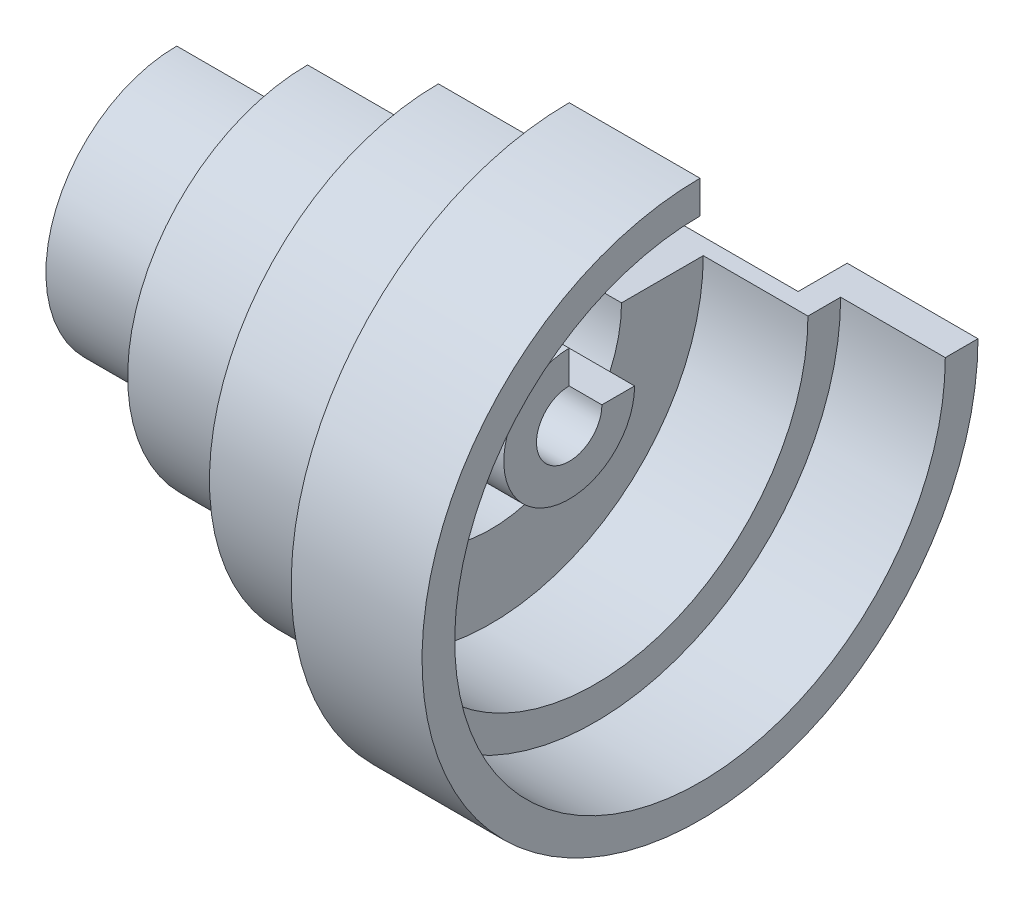
ISO-10303-21;
HEADER;
FILE_DESCRIPTION(('STEP AP214'),'2;1');
FILE_NAME('part.step','',(''),(''),'','','');
FILE_SCHEMA(('AUTOMOTIVE_DESIGN { 1 0 10303 214 1 1 1 1 }'));
ENDSEC;
DATA;
#1=APPLICATION_CONTEXT('core data for automotive mechanical design processes');
#2=APPLICATION_PROTOCOL_DEFINITION('international standard','automotive_design',2000,#1);
#3=PRODUCT_CONTEXT('',#1,'mechanical');
#4=PRODUCT('Part','Part','',(#3));
#5=PRODUCT_RELATED_PRODUCT_CATEGORY('part','',(#4));
#6=PRODUCT_DEFINITION_FORMATION('','',#4);
#7=PRODUCT_DEFINITION_CONTEXT('part definition',#1,'design');
#8=PRODUCT_DEFINITION('design','',#6,#7);
#9=PRODUCT_DEFINITION_SHAPE('','',#8);
#10=(LENGTH_UNIT() NAMED_UNIT(*) SI_UNIT(.MILLI.,.METRE.));
#11=(NAMED_UNIT(*) PLANE_ANGLE_UNIT() SI_UNIT($,.RADIAN.));
#12=(NAMED_UNIT(*) SI_UNIT($,.STERADIAN.) SOLID_ANGLE_UNIT());
#13=UNCERTAINTY_MEASURE_WITH_UNIT(LENGTH_MEASURE(1.E-05),#10,'distance_accuracy_value','');
#14=(GEOMETRIC_REPRESENTATION_CONTEXT(3) GLOBAL_UNCERTAINTY_ASSIGNED_CONTEXT((#13)) GLOBAL_UNIT_ASSIGNED_CONTEXT((#10,
#11,#12)) REPRESENTATION_CONTEXT('',''));
#15=CARTESIAN_POINT('',(0.,0.,0.));
#16=DIRECTION('',(0.,0.,1.));
#17=DIRECTION('',(1.,0.,0.));
#18=AXIS2_PLACEMENT_3D('',#15,#16,#17);
#19=CARTESIAN_POINT('',(0.,0.,0.));
#20=DIRECTION('',(-1.,0.,0.));
#21=DIRECTION('',(0.,0.,1.));
#22=AXIS2_PLACEMENT_3D('',#19,#20,#21);
#23=CYLINDRICAL_SURFACE('',#22,10.);
#24=CARTESIAN_POINT('',(120.,0.,0.));
#25=DIRECTION('',(-1.,0.,0.));
#26=DIRECTION('',(0.,0.,1.));
#27=AXIS2_PLACEMENT_3D('',#24,#25,#26);
#28=CIRCLE('',#27,10.);
#29=CARTESIAN_POINT('',(120.,1.04744440165294E-13,-10.));
#30=VERTEX_POINT('',#29);
#31=CARTESIAN_POINT('',(120.,10.,0.));
#32=VERTEX_POINT('',#31);
#33=EDGE_CURVE('E11',#30,#32,#28,.T.);
#34=ORIENTED_EDGE('',*,*,#33,.F.);
#35=DIRECTION('',(-1.,0.,0.));
#36=VECTOR('',#35,1.);
#37=CARTESIAN_POINT('',(0.,1.04744440165294E-13,-10.));
#38=LINE('',#37,#36);
#39=CARTESIAN_POINT('',(0.,1.04744440165294E-13,-10.));
#40=VERTEX_POINT('',#39);
#41=EDGE_CURVE('E228',#30,#40,#38,.T.);
#42=ORIENTED_EDGE('',*,*,#41,.T.);
#43=CARTESIAN_POINT('',(0.,0.,0.));
#44=DIRECTION('',(-1.,0.,0.));
#45=DIRECTION('',(0.,0.,1.));
#46=AXIS2_PLACEMENT_3D('',#43,#44,#45);
#47=CIRCLE('',#46,10.);
#48=CARTESIAN_POINT('',(0.,10.,0.));
#49=VERTEX_POINT('',#48);
#50=EDGE_CURVE('E57',#40,#49,#47,.T.);
#51=ORIENTED_EDGE('',*,*,#50,.T.);
#52=DIRECTION('',(-1.,0.,0.));
#53=VECTOR('',#52,1.);
#54=CARTESIAN_POINT('',(0.,10.,0.));
#55=LINE('',#54,#53);
#56=EDGE_CURVE('E178',#32,#49,#55,.T.);
#57=ORIENTED_EDGE('',*,*,#56,.F.);
#58=EDGE_LOOP('',(#34,#42,#51,#57));
#59=FACE_BOUND('',#58,.T.);
#60=ADVANCED_FACE('F41',(#59),#23,.F.);
#61=CARTESIAN_POINT('',(120.,0.,0.));
#62=DIRECTION('',(1.,0.,0.));
#63=DIRECTION('',(0.,0.,-1.));
#64=AXIS2_PLACEMENT_3D('',#61,#62,#63);
#65=PLANE('',#64);
#66=CARTESIAN_POINT('',(120.,0.,0.));
#67=DIRECTION('',(-1.,0.,0.));
#68=DIRECTION('',(0.,0.,1.));
#69=AXIS2_PLACEMENT_3D('',#66,#67,#68);
#70=CIRCLE('',#69,20.);
#71=CARTESIAN_POINT('',(120.,2.09488880330588E-13,-20.));
#72=VERTEX_POINT('',#71);
#73=CARTESIAN_POINT('',(120.,20.,0.));
#74=VERTEX_POINT('',#73);
#75=EDGE_CURVE('E47',#72,#74,#70,.T.);
#76=ORIENTED_EDGE('',*,*,#75,.F.);
#77=DIRECTION('',(0.,0.,1.));
#78=VECTOR('',#77,1.);
#79=CARTESIAN_POINT('',(120.,0.,0.));
#80=LINE('',#79,#78);
#81=EDGE_CURVE('E175',#72,#30,#80,.T.);
#82=ORIENTED_EDGE('',*,*,#81,.T.);
#83=ORIENTED_EDGE('',*,*,#33,.T.);
#84=DIRECTION('',(0.,-1.,0.));
#85=VECTOR('',#84,1.);
#86=CARTESIAN_POINT('',(120.,0.,0.));
#87=LINE('',#86,#85);
#88=EDGE_CURVE('E166',#74,#32,#87,.T.);
#89=ORIENTED_EDGE('',*,*,#88,.F.);
#90=EDGE_LOOP('',(#76,#82,#83,#89));
#91=FACE_BOUND('',#90,.T.);
#92=ADVANCED_FACE('F43',(#91),#65,.T.);
#93=CARTESIAN_POINT('',(0.,0.,0.));
#94=DIRECTION('',(-1.,0.,0.));
#95=DIRECTION('',(0.,0.,1.));
#96=AXIS2_PLACEMENT_3D('',#93,#94,#95);
#97=CYLINDRICAL_SURFACE('',#96,20.);
#98=CARTESIAN_POINT('',(63.9999999999999,0.,0.));
#99=DIRECTION('',(-1.,0.,0.));
#100=DIRECTION('',(0.,0.,1.));
#101=AXIS2_PLACEMENT_3D('',#98,#99,#100);
#102=CIRCLE('',#101,20.);
#103=CARTESIAN_POINT('',(63.9999999999999,2.09488880330588E-13,-20.));
#104=VERTEX_POINT('',#103);
#105=CARTESIAN_POINT('',(63.9999999999999,20.,0.));
#106=VERTEX_POINT('',#105);
#107=EDGE_CURVE('E307',#104,#106,#102,.T.);
#108=ORIENTED_EDGE('',*,*,#107,.F.);
#109=DIRECTION('',(1.,0.,0.));
#110=VECTOR('',#109,1.);
#111=CARTESIAN_POINT('',(0.,2.09488880330588E-13,-20.));
#112=LINE('',#111,#110);
#113=EDGE_CURVE('E232',#104,#72,#112,.T.);
#114=ORIENTED_EDGE('',*,*,#113,.T.);
#115=ORIENTED_EDGE('',*,*,#75,.T.);
#116=DIRECTION('',(1.,0.,0.));
#117=VECTOR('',#116,1.);
#118=CARTESIAN_POINT('',(0.,20.,0.));
#119=LINE('',#118,#117);
#120=EDGE_CURVE('E181',#106,#74,#119,.T.);
#121=ORIENTED_EDGE('',*,*,#120,.F.);
#122=EDGE_LOOP('',(#108,#114,#115,#121));
#123=FACE_BOUND('',#122,.T.);
#124=ADVANCED_FACE('F310',(#123),#97,.T.);
#125=CARTESIAN_POINT('',(63.9999999999999,0.,0.));
#126=DIRECTION('',(1.,0.,0.));
#127=DIRECTION('',(0.,0.,-1.));
#128=AXIS2_PLACEMENT_3D('',#125,#126,#127);
#129=PLANE('',#128);
#130=CARTESIAN_POINT('',(63.9999999999999,0.,0.));
#131=DIRECTION('',(-1.,0.,0.));
#132=DIRECTION('',(0.,0.,1.));
#133=AXIS2_PLACEMENT_3D('',#130,#131,#132);
#134=CIRCLE('',#133,40.);
#135=CARTESIAN_POINT('',(63.9999999999999,4.18977760661176E-13,-40.));
#136=VERTEX_POINT('',#135);
#137=CARTESIAN_POINT('',(63.9999999999999,40.,0.));
#138=VERTEX_POINT('',#137);
#139=EDGE_CURVE('E301',#136,#138,#134,.T.);
#140=ORIENTED_EDGE('',*,*,#139,.F.);
#141=DIRECTION('',(0.,0.,1.));
#142=VECTOR('',#141,1.);
#143=CARTESIAN_POINT('',(63.9999999999999,0.,0.));
#144=LINE('',#143,#142);
#145=EDGE_CURVE('E237',#136,#104,#144,.T.);
#146=ORIENTED_EDGE('',*,*,#145,.T.);
#147=ORIENTED_EDGE('',*,*,#107,.T.);
#148=DIRECTION('',(0.,-1.,0.));
#149=VECTOR('',#148,1.);
#150=CARTESIAN_POINT('',(63.9999999999999,0.,0.));
#151=LINE('',#150,#149);
#152=EDGE_CURVE('E183',#138,#106,#151,.T.);
#153=ORIENTED_EDGE('',*,*,#152,.F.);
#154=EDGE_LOOP('',(#140,#146,#147,#153));
#155=FACE_BOUND('',#154,.T.);
#156=ADVANCED_FACE('F370',(#155),#129,.T.);
#157=CARTESIAN_POINT('',(0.,0.,0.));
#158=DIRECTION('',(-1.,0.,0.));
#159=DIRECTION('',(0.,0.,1.));
#160=AXIS2_PLACEMENT_3D('',#157,#158,#159);
#161=CYLINDRICAL_SURFACE('',#160,40.);
#162=CARTESIAN_POINT('',(95.9999999999999,0.,0.));
#163=DIRECTION('',(-1.,0.,0.));
#164=DIRECTION('',(0.,0.,1.));
#165=AXIS2_PLACEMENT_3D('',#162,#163,#164);
#166=CIRCLE('',#165,40.);
#167=CARTESIAN_POINT('',(95.9999999999999,4.18977760661176E-13,-40.));
#168=VERTEX_POINT('',#167);
#169=CARTESIAN_POINT('',(95.9999999999999,40.,0.));
#170=VERTEX_POINT('',#169);
#171=EDGE_CURVE('E302',#168,#170,#166,.T.);
#172=ORIENTED_EDGE('',*,*,#171,.F.);
#173=DIRECTION('',(-1.,0.,0.));
#174=VECTOR('',#173,1.);
#175=CARTESIAN_POINT('',(0.,4.18977760661176E-13,-40.));
#176=LINE('',#175,#174);
#177=EDGE_CURVE('E239',#168,#136,#176,.T.);
#178=ORIENTED_EDGE('',*,*,#177,.T.);
#179=ORIENTED_EDGE('',*,*,#139,.T.);
#180=DIRECTION('',(-1.,0.,0.));
#181=VECTOR('',#180,1.);
#182=CARTESIAN_POINT('',(0.,40.,0.));
#183=LINE('',#182,#181);
#184=EDGE_CURVE('E186',#170,#138,#183,.T.);
#185=ORIENTED_EDGE('',*,*,#184,.F.);
#186=EDGE_LOOP('',(#172,#178,#179,#185));
#187=FACE_BOUND('',#186,.T.);
#188=ADVANCED_FACE('F365',(#187),#161,.F.);
#189=CARTESIAN_POINT('',(95.9999999999999,0.,0.));
#190=DIRECTION('',(1.,0.,0.));
#191=DIRECTION('',(0.,0.,-1.));
#192=AXIS2_PLACEMENT_3D('',#189,#190,#191);
#193=PLANE('',#192);
#194=CARTESIAN_POINT('',(95.9999999999999,0.,0.));
#195=DIRECTION('',(-1.,0.,0.));
#196=DIRECTION('',(0.,0.,1.));
#197=AXIS2_PLACEMENT_3D('',#194,#195,#196);
#198=CIRCLE('',#197,65.);
#199=CARTESIAN_POINT('',(95.9999999999999,6.80838861074411E-13,-65.));
#200=VERTEX_POINT('',#199);
#201=CARTESIAN_POINT('',(95.9999999999999,65.,0.));
#202=VERTEX_POINT('',#201);
#203=EDGE_CURVE('E303',#200,#202,#198,.T.);
#204=ORIENTED_EDGE('',*,*,#203,.F.);
#205=DIRECTION('',(0.,0.,1.));
#206=VECTOR('',#205,1.);
#207=CARTESIAN_POINT('',(95.9999999999999,0.,0.));
#208=LINE('',#207,#206);
#209=EDGE_CURVE('E245',#200,#168,#208,.T.);
#210=ORIENTED_EDGE('',*,*,#209,.T.);
#211=ORIENTED_EDGE('',*,*,#171,.T.);
#212=DIRECTION('',(0.,-1.,0.));
#213=VECTOR('',#212,1.);
#214=CARTESIAN_POINT('',(95.9999999999999,0.,0.));
#215=LINE('',#214,#213);
#216=EDGE_CURVE('E194',#202,#170,#215,.T.);
#217=ORIENTED_EDGE('',*,*,#216,.F.);
#218=EDGE_LOOP('',(#204,#210,#211,#217));
#219=FACE_BOUND('',#218,.T.);
#220=ADVANCED_FACE('F356',(#219),#193,.T.);
#221=CARTESIAN_POINT('',(0.,0.,0.));
#222=DIRECTION('',(-1.,0.,0.));
#223=DIRECTION('',(0.,0.,1.));
#224=AXIS2_PLACEMENT_3D('',#221,#222,#223);
#225=CYLINDRICAL_SURFACE('',#224,65.);
#226=CARTESIAN_POINT('',(128.,0.,0.));
#227=DIRECTION('',(-1.,0.,0.));
#228=DIRECTION('',(0.,0.,1.));
#229=AXIS2_PLACEMENT_3D('',#226,#227,#228);
#230=CIRCLE('',#229,65.);
#231=CARTESIAN_POINT('',(128.,6.80838861074411E-13,-65.));
#232=VERTEX_POINT('',#231);
#233=CARTESIAN_POINT('',(128.,65.,0.));
#234=VERTEX_POINT('',#233);
#235=EDGE_CURVE('E296',#232,#234,#230,.T.);
#236=ORIENTED_EDGE('',*,*,#235,.F.);
#237=DIRECTION('',(-1.,0.,0.));
#238=VECTOR('',#237,1.);
#239=CARTESIAN_POINT('',(0.,6.80838861074411E-13,-65.));
#240=LINE('',#239,#238);
#241=EDGE_CURVE('E243',#232,#200,#240,.T.);
#242=ORIENTED_EDGE('',*,*,#241,.T.);
#243=ORIENTED_EDGE('',*,*,#203,.T.);
#244=DIRECTION('',(-1.,0.,0.));
#245=VECTOR('',#244,1.);
#246=CARTESIAN_POINT('',(0.,65.,0.));
#247=LINE('',#246,#245);
#248=EDGE_CURVE('E191',#234,#202,#247,.T.);
#249=ORIENTED_EDGE('',*,*,#248,.F.);
#250=EDGE_LOOP('',(#236,#242,#243,#249));
#251=FACE_BOUND('',#250,.T.);
#252=ADVANCED_FACE('F358',(#251),#225,.F.);
#253=CARTESIAN_POINT('',(128.,0.,0.));
#254=DIRECTION('',(1.,0.,0.));
#255=DIRECTION('',(0.,0.,-1.));
#256=AXIS2_PLACEMENT_3D('',#253,#254,#255);
#257=PLANE('',#256);
#258=CARTESIAN_POINT('',(128.,0.,0.));
#259=DIRECTION('',(-1.,0.,0.));
#260=DIRECTION('',(0.,0.,1.));
#261=AXIS2_PLACEMENT_3D('',#258,#259,#260);
#262=CIRCLE('',#261,75.);
#263=CARTESIAN_POINT('',(128.,7.85583301239705E-13,-75.));
#264=VERTEX_POINT('',#263);
#265=CARTESIAN_POINT('',(128.,75.,0.));
#266=VERTEX_POINT('',#265);
#267=EDGE_CURVE('E300',#264,#266,#262,.T.);
#268=ORIENTED_EDGE('',*,*,#267,.F.);
#269=DIRECTION('',(0.,0.,1.));
#270=VECTOR('',#269,1.);
#271=CARTESIAN_POINT('',(128.,0.,0.));
#272=LINE('',#271,#270);
#273=EDGE_CURVE('E247',#264,#232,#272,.T.);
#274=ORIENTED_EDGE('',*,*,#273,.T.);
#275=ORIENTED_EDGE('',*,*,#235,.T.);
#276=DIRECTION('',(0.,-1.,0.));
#277=VECTOR('',#276,1.);
#278=CARTESIAN_POINT('',(128.,0.,0.));
#279=LINE('',#278,#277);
#280=EDGE_CURVE('E196',#266,#234,#279,.T.);
#281=ORIENTED_EDGE('',*,*,#280,.F.);
#282=EDGE_LOOP('',(#268,#274,#275,#281));
#283=FACE_BOUND('',#282,.T.);
#284=ADVANCED_FACE('F355',(#283),#257,.T.);
#285=CARTESIAN_POINT('',(0.,0.,0.));
#286=DIRECTION('',(-1.,0.,0.));
#287=DIRECTION('',(0.,0.,1.));
#288=AXIS2_PLACEMENT_3D('',#285,#286,#287);
#289=CYLINDRICAL_SURFACE('',#288,75.);
#290=CARTESIAN_POINT('',(160.,0.,0.));
#291=DIRECTION('',(-1.,0.,0.));
#292=DIRECTION('',(0.,0.,1.));
#293=AXIS2_PLACEMENT_3D('',#290,#291,#292);
#294=CIRCLE('',#293,75.);
#295=CARTESIAN_POINT('',(160.,7.85583301239705E-13,-75.));
#296=VERTEX_POINT('',#295);
#297=CARTESIAN_POINT('',(160.,75.,0.));
#298=VERTEX_POINT('',#297);
#299=EDGE_CURVE('E293',#296,#298,#294,.T.);
#300=ORIENTED_EDGE('',*,*,#299,.F.);
#301=DIRECTION('',(-1.,0.,0.));
#302=VECTOR('',#301,1.);
#303=CARTESIAN_POINT('',(0.,7.85583301239705E-13,-75.));
#304=LINE('',#303,#302);
#305=EDGE_CURVE('E253',#296,#264,#304,.T.);
#306=ORIENTED_EDGE('',*,*,#305,.T.);
#307=ORIENTED_EDGE('',*,*,#267,.T.);
#308=DIRECTION('',(-1.,0.,0.));
#309=VECTOR('',#308,1.);
#310=CARTESIAN_POINT('',(0.,75.,0.));
#311=LINE('',#310,#309);
#312=EDGE_CURVE('E203',#298,#266,#311,.T.);
#313=ORIENTED_EDGE('',*,*,#312,.F.);
#314=EDGE_LOOP('',(#300,#306,#307,#313));
#315=FACE_BOUND('',#314,.T.);
#316=ADVANCED_FACE('F346',(#315),#289,.F.);
#317=CARTESIAN_POINT('',(160.,0.,4.44089209850062E-13));
#318=DIRECTION('',(1.,0.,0.));
#319=DIRECTION('',(0.,0.,-1.));
#320=AXIS2_PLACEMENT_3D('',#317,#318,#319);
#321=PLANE('',#320);
#322=CARTESIAN_POINT('',(160.,0.,0.));
#323=DIRECTION('',(-1.,0.,0.));
#324=DIRECTION('',(0.,0.,1.));
#325=AXIS2_PLACEMENT_3D('',#322,#323,#324);
#326=CIRCLE('',#325,85.);
#327=CARTESIAN_POINT('',(160.,8.90327741404999E-13,-85.));
#328=VERTEX_POINT('',#327);
#329=CARTESIAN_POINT('',(160.,85.,0.));
#330=VERTEX_POINT('',#329);
#331=EDGE_CURVE('E291',#328,#330,#326,.T.);
#332=ORIENTED_EDGE('',*,*,#331,.F.);
#333=DIRECTION('',(0.,0.,1.));
#334=VECTOR('',#333,1.);
#335=CARTESIAN_POINT('',(160.,0.,4.44089209850062E-13));
#336=LINE('',#335,#334);
#337=EDGE_CURVE('E255',#328,#296,#336,.T.);
#338=ORIENTED_EDGE('',*,*,#337,.T.);
#339=ORIENTED_EDGE('',*,*,#299,.T.);
#340=DIRECTION('',(0.,-1.,0.));
#341=VECTOR('',#340,1.);
#342=CARTESIAN_POINT('',(160.,-4.44089209850062E-13,0.));
#343=LINE('',#342,#341);
#344=EDGE_CURVE('E204',#330,#298,#343,.T.);
#345=ORIENTED_EDGE('',*,*,#344,.F.);
#346=EDGE_LOOP('',(#332,#338,#339,#345));
#347=FACE_BOUND('',#346,.T.);
#348=ADVANCED_FACE('F345',(#347),#321,.T.);
#349=CARTESIAN_POINT('',(0.,0.,0.));
#350=DIRECTION('',(-1.,0.,0.));
#351=DIRECTION('',(0.,0.,1.));
#352=AXIS2_PLACEMENT_3D('',#349,#350,#351);
#353=CYLINDRICAL_SURFACE('',#352,85.);
#354=CARTESIAN_POINT('',(120.,0.,0.));
#355=DIRECTION('',(-1.,0.,0.));
#356=DIRECTION('',(0.,0.,1.));
#357=AXIS2_PLACEMENT_3D('',#354,#355,#356);
#358=CIRCLE('',#357,85.);
#359=CARTESIAN_POINT('',(120.,8.90327741404999E-13,-85.));
#360=VERTEX_POINT('',#359);
#361=CARTESIAN_POINT('',(120.,85.,0.));
#362=VERTEX_POINT('',#361);
#363=EDGE_CURVE('E292',#360,#362,#358,.T.);
#364=ORIENTED_EDGE('',*,*,#363,.F.);
#365=DIRECTION('',(1.,0.,0.));
#366=VECTOR('',#365,1.);
#367=CARTESIAN_POINT('',(0.,8.90327741405E-13,-85.));
#368=LINE('',#367,#366);
#369=EDGE_CURVE('E260',#360,#328,#368,.T.);
#370=ORIENTED_EDGE('',*,*,#369,.T.);
#371=ORIENTED_EDGE('',*,*,#331,.T.);
#372=DIRECTION('',(1.,0.,0.));
#373=VECTOR('',#372,1.);
#374=CARTESIAN_POINT('',(0.,85.,0.));
#375=LINE('',#374,#373);
#376=EDGE_CURVE('E210',#362,#330,#375,.T.);
#377=ORIENTED_EDGE('',*,*,#376,.F.);
#378=EDGE_LOOP('',(#364,#370,#371,#377));
#379=FACE_BOUND('',#378,.T.);
#380=ADVANCED_FACE('F338',(#379),#353,.T.);
#381=CARTESIAN_POINT('',(120.,0.,0.));
#382=DIRECTION('',(-1.,0.,0.));
#383=DIRECTION('',(0.,0.,1.));
#384=AXIS2_PLACEMENT_3D('',#381,#382,#383);
#385=PLANE('',#384);
#386=CARTESIAN_POINT('',(120.,0.,0.));
#387=DIRECTION('',(-1.,0.,0.));
#388=DIRECTION('',(0.,0.,1.));
#389=AXIS2_PLACEMENT_3D('',#386,#387,#388);
#390=CIRCLE('',#389,70.);
#391=CARTESIAN_POINT('',(120.,7.33211081157058E-13,-70.));
#392=VERTEX_POINT('',#391);
#393=CARTESIAN_POINT('',(120.,70.,0.));
#394=VERTEX_POINT('',#393);
#395=EDGE_CURVE('E290',#392,#394,#390,.T.);
#396=ORIENTED_EDGE('',*,*,#395,.F.);
#397=DIRECTION('',(0.,0.,-1.));
#398=VECTOR('',#397,1.);
#399=CARTESIAN_POINT('',(120.,0.,0.));
#400=LINE('',#399,#398);
#401=EDGE_CURVE('E257',#392,#360,#400,.T.);
#402=ORIENTED_EDGE('',*,*,#401,.T.);
#403=ORIENTED_EDGE('',*,*,#363,.T.);
#404=DIRECTION('',(0.,1.,0.));
#405=VECTOR('',#404,1.);
#406=CARTESIAN_POINT('',(120.,0.,0.));
#407=LINE('',#406,#405);
#408=EDGE_CURVE('E209',#394,#362,#407,.T.);
#409=ORIENTED_EDGE('',*,*,#408,.F.);
#410=EDGE_LOOP('',(#396,#402,#403,#409));
#411=FACE_BOUND('',#410,.T.);
#412=ADVANCED_FACE('F337',(#411),#385,.T.);
#413=CARTESIAN_POINT('',(0.,0.,0.));
#414=DIRECTION('',(-1.,0.,0.));
#415=DIRECTION('',(0.,0.,1.));
#416=AXIS2_PLACEMENT_3D('',#413,#414,#415);
#417=CYLINDRICAL_SURFACE('',#416,70.);
#418=CARTESIAN_POINT('',(80.,0.,0.));
#419=DIRECTION('',(-1.,0.,0.));
#420=DIRECTION('',(0.,0.,1.));
#421=AXIS2_PLACEMENT_3D('',#418,#419,#420);
#422=CIRCLE('',#421,70.);
#423=CARTESIAN_POINT('',(80.,7.33211081157058E-13,-70.));
#424=VERTEX_POINT('',#423);
#425=CARTESIAN_POINT('',(80.,70.,0.));
#426=VERTEX_POINT('',#425);
#427=EDGE_CURVE('E289',#424,#426,#422,.T.);
#428=ORIENTED_EDGE('',*,*,#427,.F.);
#429=DIRECTION('',(1.,0.,0.));
#430=VECTOR('',#429,1.);
#431=CARTESIAN_POINT('',(0.,7.33211081157058E-13,-70.));
#432=LINE('',#431,#430);
#433=EDGE_CURVE('E263',#424,#392,#432,.T.);
#434=ORIENTED_EDGE('',*,*,#433,.T.);
#435=ORIENTED_EDGE('',*,*,#395,.T.);
#436=DIRECTION('',(1.,0.,0.));
#437=VECTOR('',#436,1.);
#438=CARTESIAN_POINT('',(0.,70.,0.));
#439=LINE('',#438,#437);
#440=EDGE_CURVE('E213',#426,#394,#439,.T.);
#441=ORIENTED_EDGE('',*,*,#440,.F.);
#442=EDGE_LOOP('',(#428,#434,#435,#441));
#443=FACE_BOUND('',#442,.T.);
#444=ADVANCED_FACE('F335',(#443),#417,.T.);
#445=CARTESIAN_POINT('',(80.,0.,0.));
#446=DIRECTION('',(-1.,0.,0.));
#447=DIRECTION('',(0.,0.,1.));
#448=AXIS2_PLACEMENT_3D('',#445,#446,#447);
#449=PLANE('',#448);
#450=CARTESIAN_POINT('',(80.,0.,0.));
#451=DIRECTION('',(-1.,0.,0.));
#452=DIRECTION('',(0.,0.,1.));
#453=AXIS2_PLACEMENT_3D('',#450,#451,#452);
#454=CIRCLE('',#453,55.);
#455=CARTESIAN_POINT('',(80.,5.76094420909117E-13,-55.));
#456=VERTEX_POINT('',#455);
#457=CARTESIAN_POINT('',(80.,55.,0.));
#458=VERTEX_POINT('',#457);
#459=EDGE_CURVE('E283',#456,#458,#454,.T.);
#460=ORIENTED_EDGE('',*,*,#459,.F.);
#461=DIRECTION('',(0.,0.,-1.));
#462=VECTOR('',#461,1.);
#463=CARTESIAN_POINT('',(80.,0.,0.));
#464=LINE('',#463,#462);
#465=EDGE_CURVE('E266',#456,#424,#464,.T.);
#466=ORIENTED_EDGE('',*,*,#465,.T.);
#467=ORIENTED_EDGE('',*,*,#427,.T.);
#468=DIRECTION('',(0.,1.,0.));
#469=VECTOR('',#468,1.);
#470=CARTESIAN_POINT('',(80.,0.,0.));
#471=LINE('',#470,#469);
#472=EDGE_CURVE('E216',#458,#426,#471,.T.);
#473=ORIENTED_EDGE('',*,*,#472,.F.);
#474=EDGE_LOOP('',(#460,#466,#467,#473));
#475=FACE_BOUND('',#474,.T.);
#476=ADVANCED_FACE('F327',(#475),#449,.T.);
#477=CARTESIAN_POINT('',(0.,0.,0.));
#478=DIRECTION('',(-1.,0.,0.));
#479=DIRECTION('',(0.,0.,1.));
#480=AXIS2_PLACEMENT_3D('',#477,#478,#479);
#481=CYLINDRICAL_SURFACE('',#480,55.);
#482=CARTESIAN_POINT('',(40.,0.,0.));
#483=DIRECTION('',(-1.,0.,0.));
#484=DIRECTION('',(0.,0.,1.));
#485=AXIS2_PLACEMENT_3D('',#482,#483,#484);
#486=CIRCLE('',#485,55.);
#487=CARTESIAN_POINT('',(40.,5.76094420909117E-13,-55.));
#488=VERTEX_POINT('',#487);
#489=CARTESIAN_POINT('',(40.,55.,0.));
#490=VERTEX_POINT('',#489);
#491=EDGE_CURVE('E284',#488,#490,#486,.T.);
#492=ORIENTED_EDGE('',*,*,#491,.F.);
#493=DIRECTION('',(1.,0.,0.));
#494=VECTOR('',#493,1.);
#495=CARTESIAN_POINT('',(0.,5.76094420909117E-13,-55.));
#496=LINE('',#495,#494);
#497=EDGE_CURVE('E267',#488,#456,#496,.T.);
#498=ORIENTED_EDGE('',*,*,#497,.T.);
#499=ORIENTED_EDGE('',*,*,#459,.T.);
#500=DIRECTION('',(1.,0.,0.));
#501=VECTOR('',#500,1.);
#502=CARTESIAN_POINT('',(0.,55.,0.));
#503=LINE('',#502,#501);
#504=EDGE_CURVE('E218',#490,#458,#503,.T.);
#505=ORIENTED_EDGE('',*,*,#504,.F.);
#506=EDGE_LOOP('',(#492,#498,#499,#505));
#507=FACE_BOUND('',#506,.T.);
#508=ADVANCED_FACE('F322',(#507),#481,.T.);
#509=CARTESIAN_POINT('',(40.,0.,0.));
#510=DIRECTION('',(-1.,0.,0.));
#511=DIRECTION('',(0.,0.,1.));
#512=AXIS2_PLACEMENT_3D('',#509,#510,#511);
#513=PLANE('',#512);
#514=CARTESIAN_POINT('',(40.,0.,0.));
#515=DIRECTION('',(-1.,0.,0.));
#516=DIRECTION('',(0.,0.,1.));
#517=AXIS2_PLACEMENT_3D('',#514,#515,#516);
#518=CIRCLE('',#517,40.);
#519=CARTESIAN_POINT('',(40.,4.18977760661176E-13,-40.));
#520=VERTEX_POINT('',#519);
#521=CARTESIAN_POINT('',(40.,40.,0.));
#522=VERTEX_POINT('',#521);
#523=EDGE_CURVE('E282',#520,#522,#518,.T.);
#524=ORIENTED_EDGE('',*,*,#523,.F.);
#525=DIRECTION('',(0.,0.,-1.));
#526=VECTOR('',#525,1.);
#527=CARTESIAN_POINT('',(40.,0.,0.));
#528=LINE('',#527,#526);
#529=EDGE_CURVE('E275',#520,#488,#528,.T.);
#530=ORIENTED_EDGE('',*,*,#529,.T.);
#531=ORIENTED_EDGE('',*,*,#491,.T.);
#532=DIRECTION('',(0.,1.,0.));
#533=VECTOR('',#532,1.);
#534=CARTESIAN_POINT('',(40.,0.,0.));
#535=LINE('',#534,#533);
#536=EDGE_CURVE('E225',#522,#490,#535,.T.);
#537=ORIENTED_EDGE('',*,*,#536,.F.);
#538=EDGE_LOOP('',(#524,#530,#531,#537));
#539=FACE_BOUND('',#538,.T.);
#540=ADVANCED_FACE('F321',(#539),#513,.T.);
#541=CARTESIAN_POINT('',(0.,0.,0.));
#542=DIRECTION('',(-1.,0.,0.));
#543=DIRECTION('',(0.,0.,1.));
#544=AXIS2_PLACEMENT_3D('',#541,#542,#543);
#545=CYLINDRICAL_SURFACE('',#544,40.);
#546=CARTESIAN_POINT('',(0.,0.,0.));
#547=DIRECTION('',(-1.,0.,0.));
#548=DIRECTION('',(0.,0.,1.));
#549=AXIS2_PLACEMENT_3D('',#546,#547,#548);
#550=CIRCLE('',#549,40.);
#551=CARTESIAN_POINT('',(0.,4.18977760661176E-13,-40.));
#552=VERTEX_POINT('',#551);
#553=CARTESIAN_POINT('',(0.,40.,0.));
#554=VERTEX_POINT('',#553);
#555=EDGE_CURVE('E61',#552,#554,#550,.T.);
#556=ORIENTED_EDGE('',*,*,#555,.F.);
#557=DIRECTION('',(1.,0.,0.));
#558=VECTOR('',#557,1.);
#559=CARTESIAN_POINT('',(0.,4.18977760661176E-13,-40.));
#560=LINE('',#559,#558);
#561=EDGE_CURVE('E274',#552,#520,#560,.T.);
#562=ORIENTED_EDGE('',*,*,#561,.T.);
#563=ORIENTED_EDGE('',*,*,#523,.T.);
#564=DIRECTION('',(1.,0.,0.));
#565=VECTOR('',#564,1.);
#566=CARTESIAN_POINT('',(0.,40.,0.));
#567=LINE('',#566,#565);
#568=EDGE_CURVE('E223',#554,#522,#567,.T.);
#569=ORIENTED_EDGE('',*,*,#568,.F.);
#570=EDGE_LOOP('',(#556,#562,#563,#569));
#571=FACE_BOUND('',#570,.T.);
#572=ADVANCED_FACE('F320',(#571),#545,.T.);
#573=CARTESIAN_POINT('',(0.,0.,0.));
#574=DIRECTION('',(-1.,0.,0.));
#575=DIRECTION('',(0.,0.,1.));
#576=AXIS2_PLACEMENT_3D('',#573,#574,#575);
#577=PLANE('',#576);
#578=DIRECTION('',(0.,0.,-1.));
#579=VECTOR('',#578,1.);
#580=CARTESIAN_POINT('',(0.,0.,0.));
#581=LINE('',#580,#579);
#582=EDGE_CURVE('E280',#40,#552,#581,.T.);
#583=ORIENTED_EDGE('',*,*,#582,.T.);
#584=ORIENTED_EDGE('',*,*,#555,.T.);
#585=DIRECTION('',(0.,1.,0.));
#586=VECTOR('',#585,1.);
#587=CARTESIAN_POINT('',(0.,0.,0.));
#588=LINE('',#587,#586);
#589=EDGE_CURVE('E229',#49,#554,#588,.T.);
#590=ORIENTED_EDGE('',*,*,#589,.F.);
#591=ORIENTED_EDGE('',*,*,#50,.F.);
#592=EDGE_LOOP('',(#583,#584,#590,#591));
#593=FACE_BOUND('',#592,.T.);
#594=ADVANCED_FACE('F316',(#593),#577,.T.);
#595=CARTESIAN_POINT('',(0.,0.,0.));
#596=DIRECTION('',(0.,1.,0.));
#597=DIRECTION('',(1.,0.,0.));
#598=AXIS2_PLACEMENT_3D('',#595,#596,#597);
#599=PLANE('',#598);
#600=ORIENTED_EDGE('',*,*,#41,.F.);
#601=ORIENTED_EDGE('',*,*,#81,.F.);
#602=ORIENTED_EDGE('',*,*,#113,.F.);
#603=ORIENTED_EDGE('',*,*,#145,.F.);
#604=ORIENTED_EDGE('',*,*,#177,.F.);
#605=ORIENTED_EDGE('',*,*,#209,.F.);
#606=ORIENTED_EDGE('',*,*,#241,.F.);
#607=ORIENTED_EDGE('',*,*,#273,.F.);
#608=ORIENTED_EDGE('',*,*,#305,.F.);
#609=ORIENTED_EDGE('',*,*,#337,.F.);
#610=ORIENTED_EDGE('',*,*,#369,.F.);
#611=ORIENTED_EDGE('',*,*,#401,.F.);
#612=ORIENTED_EDGE('',*,*,#433,.F.);
#613=ORIENTED_EDGE('',*,*,#465,.F.);
#614=ORIENTED_EDGE('',*,*,#497,.F.);
#615=ORIENTED_EDGE('',*,*,#529,.F.);
#616=ORIENTED_EDGE('',*,*,#561,.F.);
#617=ORIENTED_EDGE('',*,*,#582,.F.);
#618=EDGE_LOOP('',(#600,#601,#602,#603,#604,#605,#606,#607,#608,#609,#610,#611,#612,#613,#614,
#615,#616,#617));
#619=FACE_BOUND('',#618,.T.);
#620=ADVANCED_FACE('F315',(#619),#599,.T.);
#621=CARTESIAN_POINT('',(0.,0.,0.));
#622=DIRECTION('',(0.,0.,1.));
#623=DIRECTION('',(1.,0.,0.));
#624=AXIS2_PLACEMENT_3D('',#621,#622,#623);
#625=PLANE('',#624);
#626=ORIENTED_EDGE('',*,*,#56,.T.);
#627=ORIENTED_EDGE('',*,*,#589,.T.);
#628=ORIENTED_EDGE('',*,*,#568,.T.);
#629=ORIENTED_EDGE('',*,*,#536,.T.);
#630=ORIENTED_EDGE('',*,*,#504,.T.);
#631=ORIENTED_EDGE('',*,*,#472,.T.);
#632=ORIENTED_EDGE('',*,*,#440,.T.);
#633=ORIENTED_EDGE('',*,*,#408,.T.);
#634=ORIENTED_EDGE('',*,*,#376,.T.);
#635=ORIENTED_EDGE('',*,*,#344,.T.);
#636=ORIENTED_EDGE('',*,*,#312,.T.);
#637=ORIENTED_EDGE('',*,*,#280,.T.);
#638=ORIENTED_EDGE('',*,*,#248,.T.);
#639=ORIENTED_EDGE('',*,*,#216,.T.);
#640=ORIENTED_EDGE('',*,*,#184,.T.);
#641=ORIENTED_EDGE('',*,*,#152,.T.);
#642=ORIENTED_EDGE('',*,*,#120,.T.);
#643=ORIENTED_EDGE('',*,*,#88,.T.);
#644=EDGE_LOOP('',(#626,#627,#628,#629,#630,#631,#632,#633,#634,#635,#636,#637,#638,#639,#640,
#641,#642,#643));
#645=FACE_BOUND('',#644,.T.);
#646=ADVANCED_FACE('F176',(#645),#625,.F.);
#647=CLOSED_SHELL('',(#60,#92,#124,#156,#188,#220,#252,#284,#316,#348,#380,#412,#444,#476,#508,
#540,#572,#594,#620,#646));
#648=MANIFOLD_SOLID_BREP('B2',#647);
#649=ADVANCED_BREP_SHAPE_REPRESENTATION('',(#18,#648),#14);
#650=SHAPE_DEFINITION_REPRESENTATION(#9,#649);
ENDSEC;
END-ISO-10303-21;
